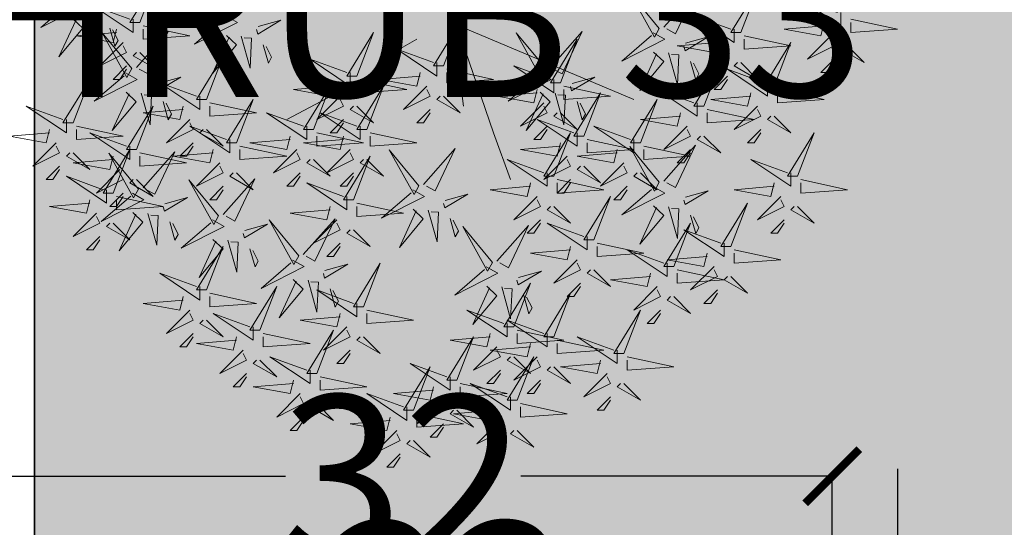
# Model space of a CAD drawing. Units: inches. Extents: x 1704 to 6393, y -157 to 1172.
# Tile 12 of 122: x 1898 to 1934, y 120 to 138. Entities that reach past the tile are written whole.
import ezdxf

# ---------------------------------------------------------------- set-up
doc = ezdxf.new("R2010")
doc.units = ezdxf.units.IN
doc.header["$MEASUREMENT"] = 0
for name, color, linetype, lineweight in [('A-ANNO-DIMS', 7, 'Continuous', 13), ('C-PROP', 7, 'Continuous', 35), ('L-shrub', 74, 'Continuous', 18)]:
    doc.layers.add(name, color=color, linetype=linetype, lineweight=lineweight)
doc.layers.add('L-PLNT-PATT', color=253, linetype='Continuous', lineweight=13, true_color=0x9abc8f)
doc.styles.get("Standard").update_dxf_attribs({"font": 'arial.ttf'})
doc.dimstyles.get("Standard").update_dxf_attribs({"dimtxt": 6, "dimasz": 2, "dimexe": 0.18, "dimexo": 0.0625, "dimgap": 0.09, "dimtad": 0, "dimtih": 1, "dimtoh": 1, "dimdec": 1, "dimzin": 0, "dimdsep": 46, "dimlunit": 3, "dimtxsty": 'Standard', "dimblk": 'ARCHTICK', "dimcen": 0.09, "dimadec": 0, "dimazin": 0, "dimtfac": 1, "dimtdec": 1, "dimtofl": 0, "dimtmove": 0, "dimatfit": 3, "dimfxl": 1, "dimtolj": 1, "dimtzin": 0, "dimarcsym": 0})

# ---------------------------------------------------------------- blocks, each defined once
blk = doc.blocks.new('autumn shrub')
at = {"layer": 'L-shrub'}
for p, q in [((11.54, 1.92), (51.94, 98)), ((71.18, 17.29), (98.12, 26.9)), ((9.62, -3.84), (71.18, 17.29)), ((11.54, -5.76), (55.79, 0)), ((17.31, -26.9), (25.01, -40.35)), ((46.17, -69.17), (63.49, -101.84))]:
    blk.add_line(p, q, dxfattribs=at)
for points in [[(5.77, 222.89), (11.54, 249.79), (13.47, 222.89), (7.7, 222.89)], [(21.16, 220.97), (30.78, 230.58), (23.09, 217.13), (21.16, 219.05)], [(1.92, 217.13), (9.62, 217.13), (-5.77, 194.07), (1.92, 215.21)], [(98.12, 194.07), (103.89, 220.97), (105.81, 194.07), (100.04, 194.07)], [(15.39, 211.36), (28.86, 197.91), (21.16, 213.28), (17.31, 211.36)], [(28.86, 213.28), (36.55, 205.6), (36.55, 209.44), (30.78, 213.28)], [(7.7, 207.52), (15.39, 205.6), (11.54, 184.46), (9.62, 207.52)], [(46.17, 180.62), (51.94, 207.52), (53.87, 180.62), (48.1, 180.62)], [(96.19, 192.15), (71.18, 201.75), (96.19, 186.38), (96.19, 192.15)], [(113.51, 192.15), (123.13, 201.75), (115.43, 188.3), (113.51, 190.23)], [(15.39, 161.4), (21.16, 188.3), (23.09, 161.4), (17.31, 161.4)], [(44.25, 178.7), (19.24, 188.3), (44.25, 172.93), (44.25, 178.7)], [(61.56, 178.7), (71.18, 188.3), (63.49, 174.85), (61.56, 176.78)], [(94.27, 188.3), (101.96, 188.3), (86.57, 165.25), (94.27, 186.38)], [(107.74, 182.54), (121.2, 169.09), (113.51, 184.46), (109.66, 182.54)], [(121.2, 184.46), (128.9, 176.78), (128.9, 180.62), (123.13, 184.46)], [(138.52, 155.64), (144.29, 182.54), (146.21, 155.64), (140.44, 155.64)], [(100.04, 178.7), (107.74, 176.78), (103.89, 155.64), (101.96, 178.7)], [(42.32, 174.85), (50.02, 174.85), (34.63, 151.8), (42.32, 172.93)], [(55.79, 169.09), (69.26, 155.64), (61.56, 171.01), (57.72, 169.09)], [(69.26, 171.01), (76.95, 163.33), (76.95, 167.17), (71.18, 171.01)], [(13.47, 159.48), (-11.54, 169.09), (13.47, 153.72), (13.47, 159.48)], [(30.78, 159.48), (40.4, 169.09), (32.71, 155.64), (30.78, 157.56)], [(48.1, 165.25), (55.79, 163.33), (51.94, 142.19), (50.02, 165.25)], [(57.72, 140.27), (63.49, 167.17), (65.41, 140.27), (59.64, 140.27)], [(136.59, 153.72), (111.58, 163.33), (136.59, 147.95), (136.59, 153.72)], [(153.91, 153.72), (163.53, 163.33), (155.83, 149.87), (153.91, 151.8)], [(11.54, 155.64), (19.24, 155.64), (3.85, 132.58), (11.54, 153.72)], [(25.01, 149.87), (38.48, 136.42), (30.78, 151.8), (26.93, 149.87)], [(55.79, 138.35), (30.78, 147.95), (55.79, 132.58), (55.79, 138.35)], [(38.48, 151.8), (46.17, 144.11), (46.17, 147.95), (40.4, 151.8)], [(73.11, 138.35), (82.73, 147.95), (75.03, 134.5), (73.11, 136.42)], [(134.67, 149.87), (142.36, 149.87), (126.97, 126.82), (134.67, 147.95)], [(150.06, 122.97), (155.83, 149.87), (157.76, 122.97), (151.98, 122.97)], [(17.31, 146.03), (25.01, 144.11), (21.16, 122.97), (19.24, 146.03)], [(148.14, 144.11), (161.6, 130.66), (153.91, 146.03), (150.06, 144.11)], [(161.6, 146.03), (169.3, 138.35), (169.3, 142.19), (163.53, 146.03)], [(19.67, 127.72), (16.03, 140.82), (23.96, 127.51), (21.35, 126.78)], [(108.17, 127.72), (104.53, 140.82), (112.46, 127.51), (109.84, 126.78)], [(140.44, 140.27), (148.14, 138.35), (144.29, 117.21), (142.36, 140.27)], [(10.44, 115.26), (-10.16, 133.5), (14.22, 121.96), (11.38, 116.94)], [(30.15, 130.65), (40.62, 133.58), (37.28, 135.46), (31.09, 132.32)], [(53.87, 134.5), (61.56, 134.5), (46.17, 111.45), (53.87, 132.58)], [(67.33, 128.74), (80.8, 115.29), (73.11, 130.66), (69.26, 128.74)], [(98.93, 115.26), (78.34, 133.5), (102.71, 121.96), (99.88, 116.94)], [(78.88, 103.76), (84.65, 130.66), (86.57, 103.76), (80.8, 103.76)], [(80.8, 130.66), (88.5, 122.97), (88.5, 126.82), (82.73, 130.66)], [(118.64, 130.65), (129.12, 133.58), (125.77, 135.46), (119.59, 132.32)], [(148.14, 121.05), (123.13, 130.66), (148.14, 115.29), (148.14, 121.05)], [(165.45, 121.05), (175.07, 130.66), (167.38, 117.21), (165.45, 119.13)], [(59.64, 124.9), (67.33, 122.97), (63.49, 101.84), (61.56, 124.9)], [(25.2, 117.98), (43.54, 123.1), (26.37, 123.95), (26.15, 119.65)], [(113.7, 117.98), (132.03, 123.1), (114.86, 123.95), (114.65, 119.65)], [(200.08, 94.15), (205.85, 121.05), (207.78, 94.15), (202, 94.15)], [(13.57, 109.08), (17.35, 115.78), (29.87, 91.05), (15.24, 108.13)], [(24.77, 109.38), (30.23, 115.14), (46.74, 101.41), (25.72, 111.06)], [(102.06, 109.08), (105.85, 115.78), (118.37, 91.05), (103.74, 108.13)], [(113.27, 109.38), (118.72, 115.14), (135.24, 101.41), (114.21, 111.06)], [(146.21, 117.21), (153.91, 117.21), (138.52, 94.15), (146.21, 115.29)], [(159.68, 111.45), (173.15, 98), (165.45, 113.37), (161.6, 111.45)], [(173.15, 113.37), (180.84, 105.68), (180.84, 109.52), (175.07, 113.37)], [(11.17, 112.64), (-9.49, 95.58), (16.19, 109.81), (11.17, 112.64)], [(76.95, 101.84), (51.94, 111.45), (76.95, 96.07), (76.95, 101.84)], [(99.66, 112.64), (79.01, 95.58), (104.68, 109.81), (99.66, 112.64)], [(94.27, 101.84), (103.89, 111.45), (96.19, 98), (94.27, 99.92)], [(134.67, 76.86), (140.44, 103.76), (142.36, 76.86), (136.59, 76.86)], [(151.98, 107.6), (159.68, 105.68), (155.83, 84.54), (153.91, 107.6)], [(75.03, 98), (82.73, 98), (67.33, 74.94), (75.03, 96.07)], [(75.03, 71.09), (80.8, 98), (82.73, 71.09), (76.95, 71.09)], [(198.16, 92.23), (173.15, 101.84), (198.16, 86.47), (198.16, 92.23)], [(215.47, 92.23), (225.09, 101.84), (217.4, 88.39), (215.47, 90.31)], [(88.5, 92.23), (101.96, 78.78), (94.27, 94.15), (90.42, 92.23)], [(101.96, 94.15), (109.66, 86.47), (109.66, 90.31), (103.89, 94.15)], [(80.8, 88.39), (88.5, 86.47), (84.65, 65.33), (82.73, 88.39)], [(196.23, 88.39), (203.93, 88.39), (188.54, 65.33), (196.23, 86.47)], [(44.25, 57.64), (50.02, 84.54), (51.94, 57.64), (46.17, 57.64)], [(98.12, 53.8), (103.89, 80.7), (105.81, 53.8), (100.04, 53.8)], [(132.75, 74.94), (107.74, 84.54), (132.75, 69.17), (132.75, 74.94)], [(150.06, 74.94), (159.68, 84.54), (151.98, 71.09), (150.06, 73.02)], [(190.46, 53.8), (196.23, 80.7), (198.16, 53.8), (192.39, 53.8)], [(209.7, 82.62), (223.17, 69.17), (215.47, 84.54), (211.62, 82.62)], [(223.17, 84.54), (230.86, 76.86), (230.86, 80.7), (225.09, 84.54)], [(42.76, 62.39), (39.12, 75.49), (47.05, 62.18), (44.43, 61.45)], [(73.11, 69.17), (48.1, 78.78), (73.11, 63.41), (73.11, 69.17)], [(90.42, 69.17), (100.04, 78.78), (92.34, 65.33), (90.42, 67.25)], [(202, 78.78), (209.7, 76.86), (205.85, 55.72), (203.93, 78.78)], [(33.52, 49.93), (12.93, 68.17), (37.3, 56.63), (34.47, 51.61)], [(53.23, 65.32), (63.71, 68.25), (60.36, 70.13), (54.18, 66.99)], [(130.82, 71.09), (138.52, 71.09), (123.13, 48.04), (130.82, 69.17)], [(42.32, 55.72), (17.31, 65.33), (42.32, 49.96), (42.32, 55.72)], [(59.64, 55.72), (69.26, 65.33), (61.56, 51.88), (59.64, 53.8)], [(71.18, 65.33), (78.88, 65.33), (63.49, 42.27), (71.18, 63.41)], [(144.29, 65.33), (157.76, 51.88), (150.06, 67.25), (146.21, 65.33)], [(157.76, 67.25), (165.45, 59.57), (165.45, 63.41), (159.68, 67.25)], [(48.29, 52.64), (66.62, 57.77), (49.45, 58.62), (49.24, 54.32)], [(96.19, 51.88), (71.18, 61.49), (96.19, 46.12), (96.19, 51.88)], [(84.65, 59.57), (98.12, 46.12), (90.42, 61.49), (86.57, 59.57)], [(98.12, 61.49), (105.81, 53.8), (105.81, 57.64), (100.04, 61.49)], [(113.51, 51.88), (123.13, 61.49), (115.43, 48.04), (113.51, 49.96)], [(136.59, 61.49), (144.29, 59.57), (140.44, 38.43), (138.52, 61.49)], [(188.54, 51.88), (163.53, 61.49), (188.54, 46.12), (188.54, 51.88)], [(184.69, 30.74), (190.46, 57.64), (192.39, 30.74), (186.61, 30.74)], [(205.85, 51.88), (215.47, 61.49), (207.78, 48.04), (205.85, 49.96)], [(227.01, 32.67), (232.79, 59.57), (234.71, 32.67), (228.94, 32.67)], [(40.4, 51.88), (48.1, 51.88), (32.71, 28.82), (40.4, 49.96)], [(76.95, 55.72), (84.65, 53.8), (80.8, 32.67), (78.88, 55.72)], [(34.25, 47.31), (13.6, 30.25), (39.27, 44.48), (34.25, 47.31)], [(36.65, 43.75), (40.43, 50.45), (52.96, 25.72), (38.33, 42.8)], [(47.86, 44.05), (53.31, 49.81), (69.83, 36.08), (48.8, 45.73)], [(53.87, 46.12), (67.33, 32.67), (59.64, 48.04), (55.79, 46.12)], [(67.33, 48.04), (75.03, 40.35), (75.03, 44.19), (69.26, 48.04)], [(94.27, 48.04), (101.96, 48.04), (86.57, 24.98), (94.27, 46.12)], [(186.61, 48.04), (194.31, 48.04), (178.92, 24.98), (186.61, 46.12)], [(46.17, 42.27), (53.87, 40.35), (50.02, 19.21), (48.1, 42.27)], [(107.74, 42.27), (121.2, 28.82), (113.51, 44.19), (109.66, 42.27)], [(121.2, 44.19), (128.9, 36.51), (128.9, 40.35), (123.13, 44.19)], [(154.34, 31.65), (150.7, 44.75), (158.63, 31.44), (156.02, 30.7)], [(200.08, 42.27), (213.55, 28.82), (205.85, 44.19), (202, 42.27)], [(225.09, 30.74), (200.08, 40.35), (225.09, 24.98), (225.09, 30.74)], [(213.55, 44.19), (221.24, 36.51), (221.24, 40.35), (215.47, 44.19)], [(242.41, 30.74), (252.02, 40.35), (244.33, 26.9), (242.41, 28.82)], [(100.04, 38.43), (107.74, 36.51), (103.89, 15.37), (101.96, 38.43)], [(145.11, 19.19), (124.51, 37.43), (148.89, 25.89), (146.05, 20.86)], [(182.77, 28.82), (157.76, 38.43), (182.77, 23.06), (182.77, 28.82)], [(164.82, 34.57), (175.29, 37.5), (171.94, 39.39), (165.76, 36.25)], [(192.39, 38.43), (200.08, 36.51), (196.23, 15.37), (194.31, 38.43)], [(200.08, 28.82), (209.7, 38.43), (202, 24.98), (200.08, 26.9)], [(159.87, 21.9), (178.21, 27.02), (161.04, 27.87), (160.82, 23.58)], [(180.84, 24.98), (188.54, 24.98), (173.15, 1.92), (180.84, 23.06)], [(223.17, 26.9), (230.86, 26.9), (215.47, 3.84), (223.17, 24.98)], [(215.47, -1.92), (221.24, 24.98), (223.17, -1.92), (217.4, -1.92)], [(236.63, 21.14), (250.1, 7.69), (242.41, 23.06), (238.56, 21.14)], [(250.1, 23.06), (257.8, 15.37), (257.8, 19.21), (252.02, 23.06)], [(34.63, -9.61), (40.4, 17.29), (42.32, -9.61), (36.55, -9.61)], [(148.24, 13), (152.02, 19.71), (164.54, -5.03), (149.91, 12.06)], [(159.44, 13.31), (164.89, 19.07), (181.41, 5.33), (160.39, 14.99)], [(194.31, 19.21), (207.78, 5.76), (200.08, 21.14), (196.23, 19.21)], [(207.78, 21.14), (215.47, 13.45), (215.47, 17.29), (209.7, 21.14)], [(228.94, 17.29), (236.63, 15.37), (232.79, -5.76), (230.86, 17.29)], [(145.83, 16.57), (125.18, -0.5), (150.86, 13.74), (145.83, 16.57)], [(186.61, 15.37), (194.31, 13.45), (190.46, -7.69), (188.54, 15.37)], [(213.55, -3.84), (188.54, 5.76), (213.55, -9.61), (213.55, -3.84)], [(230.86, -3.84), (240.48, 5.76), (232.79, -7.69), (230.86, -5.76)], [(110.09, -10.62), (106.45, 2.47), (114.39, -10.84), (111.77, -11.57)], [(232.79, -26.9), (238.56, 0), (240.48, -26.9), (234.71, -26.9)], [(32.71, -11.53), (7.7, -1.92), (32.71, -17.29), (32.71, -11.53)], [(50.02, -11.53), (59.64, -1.92), (51.94, -15.37), (50.02, -13.45)], [(100.86, -23.09), (80.26, -4.84), (104.64, -16.38), (101.8, -21.41)], [(120.57, -7.7), (131.04, -4.77), (127.7, -2.88), (121.51, -6.02)], [(211.62, -7.69), (219.32, -7.69), (203.93, -30.74), (211.62, -9.61)], [(30.78, -15.37), (38.48, -15.37), (23.09, -38.43), (30.78, -17.29)], [(115.63, -20.37), (133.96, -15.25), (116.79, -14.4), (116.57, -18.7)], [(225.09, -13.45), (238.56, -26.9), (230.86, -11.53), (227.01, -13.45)], [(238.56, -11.53), (246.25, -19.21), (246.25, -15.37), (240.48, -11.53)], [(44.25, -21.14), (57.72, -34.59), (50.02, -19.21), (46.17, -21.14)], [(57.72, -19.21), (65.41, -26.9), (65.41, -23.06), (59.64, -19.21)], [(103.99, -29.27), (107.77, -22.57), (120.29, -47.3), (105.66, -30.21)], [(230.86, -28.82), (205.85, -19.21), (230.86, -34.59), (230.86, -28.82)], [(217.4, -17.29), (225.09, -19.21), (221.24, -40.35), (219.32, -17.29)], [(248.18, -28.82), (257.8, -19.21), (250.1, -32.67), (248.18, -30.74)], [(36.55, -24.98), (44.25, -26.9), (40.4, -48.04), (38.48, -24.98)], [(71.18, -53.8), (76.95, -26.9), (78.88, -53.8), (73.11, -53.8)], [(101.59, -25.71), (80.93, -42.77), (106.61, -28.54), (101.59, -25.71)], [(115.19, -28.96), (120.65, -23.2), (137.17, -36.94), (116.14, -27.29)], [(40.4, -59.57), (46.17, -32.67), (48.1, -59.57), (42.32, -59.57)], [(173.15, -55.72), (178.92, -28.82), (180.84, -55.72), (175.07, -55.72)], [(228.94, -32.67), (236.63, -32.67), (221.24, -55.72), (228.94, -34.59)], [(111.58, -61.49), (117.35, -34.59), (119.28, -61.49), (113.51, -61.49)], [(242.41, -38.43), (255.87, -51.88), (248.18, -36.51), (244.33, -38.43)], [(255.87, -36.51), (263.57, -44.19), (263.57, -40.35), (257.8, -36.51)], [(234.71, -42.27), (242.41, -44.19), (238.56, -65.33), (236.63, -42.27)], [(69.26, -55.72), (44.25, -46.12), (69.26, -61.49), (69.26, -55.72)], [(86.57, -55.72), (96.19, -46.12), (88.5, -59.57), (86.57, -57.64)], [(171.22, -57.64), (146.21, -48.04), (171.22, -63.41), (171.22, -57.64)], [(188.54, -57.64), (198.16, -48.04), (190.46, -61.49), (188.54, -59.57)], [(38.48, -61.49), (13.47, -51.88), (38.48, -67.25), (38.48, -61.49)], [(55.79, -61.49), (65.41, -51.88), (57.72, -65.33), (55.79, -63.41)], [(109.66, -63.41), (84.65, -53.8), (109.66, -69.17), (109.66, -63.41)], [(126.97, -63.41), (136.59, -53.8), (128.9, -67.25), (126.97, -65.33)], [(211.62, -82.62), (217.4, -55.72), (219.32, -82.62), (213.55, -82.62)], [(67.33, -59.57), (75.03, -59.57), (59.64, -82.62), (67.33, -61.49)], [(71.18, -84.54), (76.95, -57.64), (78.88, -84.54), (73.11, -84.54)], [(169.3, -61.49), (176.99, -61.49), (161.6, -84.54), (169.3, -63.41)], [(36.55, -65.33), (44.25, -65.33), (28.86, -88.39), (36.55, -67.25)], [(80.8, -65.33), (94.27, -78.78), (86.57, -63.41), (82.73, -65.33)], [(94.27, -63.41), (101.96, -71.09), (101.96, -67.25), (96.19, -63.41)], [(107.74, -67.25), (115.43, -67.25), (100.04, -90.31), (107.74, -69.17)], [(150.49, -79.8), (146.85, -66.7), (154.79, -80.01), (152.17, -80.74)], [(182.77, -67.25), (196.23, -80.7), (188.54, -65.33), (184.69, -67.25)], [(196.23, -65.33), (203.93, -73.02), (203.93, -69.17), (198.16, -65.33)], [(50.02, -71.09), (63.49, -84.54), (55.79, -69.17), (51.94, -71.09)], [(63.49, -69.17), (71.18, -76.86), (71.18, -73.02), (65.41, -69.17)], [(73.11, -69.17), (80.8, -71.09), (76.95, -92.23), (75.03, -69.17)], [(121.2, -73.02), (134.67, -86.47), (126.97, -71.09), (123.13, -73.02)], [(134.67, -71.09), (142.36, -78.78), (142.36, -74.94), (136.59, -71.09)], [(160.97, -76.87), (171.44, -73.94), (168.1, -72.06), (161.91, -75.19)], [(175.07, -71.09), (182.77, -73.02), (178.92, -94.15), (176.99, -71.09)], [(42.32, -74.94), (50.02, -76.86), (46.17, -98), (44.25, -74.94)], [(69.26, -86.47), (44.25, -76.86), (69.26, -92.23), (69.26, -86.47)], [(86.57, -86.47), (96.19, -76.86), (88.5, -90.31), (86.57, -88.39)], [(113.51, -76.86), (121.2, -78.78), (117.35, -99.92), (115.43, -76.86)], [(141.26, -92.26), (120.66, -74.02), (145.04, -85.56), (142.2, -90.58)], [(209.7, -84.54), (184.69, -74.94), (209.7, -90.31), (209.7, -84.54)], [(227.01, -84.54), (236.63, -74.94), (228.94, -88.39), (227.01, -86.47)], [(156.03, -89.54), (174.36, -84.42), (157.19, -83.57), (156.97, -87.87)], [(67.33, -90.31), (75.03, -90.31), (59.64, -113.37), (67.33, -92.23)], [(186.61, -115.29), (192.39, -88.39), (194.31, -115.29), (188.54, -115.29)], [(207.78, -88.39), (215.47, -88.39), (200.08, -111.45), (207.78, -90.31)], [(80.8, -96.07), (94.27, -109.52), (86.57, -94.15), (82.73, -96.07)], [(94.27, -94.15), (101.96, -101.84), (101.96, -98), (96.19, -94.15)], [(141.99, -94.88), (121.33, -111.94), (147.01, -97.71), (141.99, -94.88)], [(144.39, -98.44), (148.17, -91.74), (160.69, -116.47), (146.06, -99.39)], [(155.59, -98.13), (161.05, -92.38), (177.57, -106.11), (156.54, -96.46)], [(221.24, -94.15), (234.71, -107.6), (227.01, -92.23), (223.17, -94.15)], [(234.71, -92.23), (242.41, -99.92), (242.41, -96.07), (236.63, -92.23)], [(73.11, -99.92), (80.8, -101.84), (76.95, -122.97), (75.03, -99.92)], [(78.88, -128.74), (84.65, -101.84), (86.57, -128.74), (80.8, -128.74)], [(213.55, -98), (221.24, -99.92), (217.4, -121.05), (215.47, -98)], [(10.05, -118.23), (6.41, -105.13), (14.35, -118.44), (11.73, -119.17)], [(184.69, -117.21), (159.68, -107.6), (184.69, -122.97), (184.69, -117.21)], [(202, -117.21), (211.62, -107.6), (203.93, -121.05), (202, -119.13)], [(20.53, -115.3), (31, -112.37), (27.66, -110.49), (21.47, -113.62)], [(127.41, -125.91), (123.77, -112.81), (131.7, -126.12), (129.08, -126.86)], [(137.88, -122.99), (148.36, -120.06), (145.01, -118.17), (138.83, -121.31)], [(15.59, -127.97), (33.92, -122.85), (16.75, -122), (16.53, -126.3)], [(76.95, -130.66), (51.94, -121.05), (76.95, -136.42), (76.95, -130.66)], [(53.87, -146.03), (59.64, -119.13), (61.56, -146.03), (55.79, -146.03)], [(94.27, -130.66), (103.89, -121.05), (96.19, -134.5), (94.27, -132.58)], [(118.17, -138.37), (97.58, -120.13), (121.95, -131.67), (119.12, -136.7)], [(163.53, -146.03), (169.3, -119.13), (171.22, -146.03), (165.45, -146.03)], [(182.77, -121.05), (190.46, -121.05), (175.07, -144.11), (182.77, -122.97)], [(3.95, -136.87), (7.73, -130.17), (20.25, -154.9), (5.62, -137.82)], [(132.94, -135.66), (151.27, -130.54), (134.1, -129.69), (133.89, -133.98)], [(196.23, -126.82), (209.7, -140.27), (202, -124.9), (198.16, -126.82)], [(209.7, -124.9), (217.4, -132.58), (217.4, -128.74), (211.62, -124.9)], [(1.55, -133.31), (-19.11, -150.37), (6.57, -136.14), (1.55, -133.31)], [(15.15, -136.56), (20.61, -130.81), (37.13, -144.54), (16.1, -134.89)], [(75.03, -134.5), (82.73, -134.5), (67.33, -157.56), (75.03, -136.42)], [(188.54, -130.66), (196.23, -132.58), (192.39, -153.72), (190.46, -130.66)], [(51.94, -147.95), (26.93, -138.35), (51.94, -153.72), (51.94, -147.95)], [(69.26, -147.95), (78.88, -138.35), (71.18, -151.8), (69.26, -149.87)], [(88.5, -140.27), (101.96, -153.72), (94.27, -138.35), (90.42, -140.27)], [(118.9, -140.99), (98.25, -158.06), (123.92, -143.83), (118.9, -140.99)], [(101.96, -138.35), (109.66, -146.03), (109.66, -142.19), (103.89, -138.35)], [(121.3, -144.56), (125.08, -137.85), (137.61, -162.59), (122.98, -145.5)], [(132.51, -144.25), (137.96, -138.49), (154.48, -152.23), (133.45, -142.57)], [(161.6, -147.95), (136.59, -138.35), (161.6, -153.72), (161.6, -147.95)], [(178.92, -147.95), (188.54, -138.35), (180.84, -151.8), (178.92, -149.87)], [(80.8, -144.11), (88.5, -146.03), (84.65, -167.17), (82.73, -144.11)], [(50.02, -151.8), (57.72, -151.8), (42.32, -174.85), (50.02, -153.72)], [(159.68, -151.8), (167.38, -151.8), (151.98, -174.85), (159.68, -153.72)], [(9.62, -184.46), (15.39, -157.56), (17.31, -184.46), (11.54, -184.46)], [(63.49, -157.56), (76.95, -171.01), (69.26, -155.64), (65.41, -157.56)], [(76.95, -155.64), (84.65, -163.33), (84.65, -159.48), (78.88, -155.64)], [(173.15, -157.56), (186.61, -171.01), (178.92, -155.64), (175.07, -157.56)], [(186.61, -155.64), (194.31, -163.33), (194.31, -159.48), (188.54, -155.64)], [(42.76, -175.87), (39.12, -162.77), (47.05, -176.08), (44.43, -176.81)], [(55.79, -161.4), (63.49, -163.33), (59.64, -184.46), (57.72, -161.4)], [(82.73, -186.38), (88.5, -159.48), (90.42, -186.38), (84.65, -186.38)], [(112.02, -172.03), (108.37, -158.93), (116.31, -172.24), (113.69, -172.97)], [(122.49, -169.1), (132.97, -166.17), (129.62, -164.29), (123.44, -167.43)], [(165.45, -161.4), (173.15, -163.33), (169.3, -184.46), (167.38, -161.4)], [(53.23, -172.94), (63.71, -170.02), (60.36, -168.13), (54.18, -171.27)], [(102.78, -184.49), (82.19, -166.25), (106.56, -177.79), (103.73, -182.81)], [(33.52, -188.33), (12.93, -170.09), (37.3, -181.63), (34.47, -186.66)], [(107.74, -199.83), (113.51, -172.93), (115.43, -199.83), (109.66, -199.83)], [(7.7, -186.38), (-17.31, -176.78), (7.7, -192.15), (7.7, -186.38)], [(25.01, -186.38), (34.63, -176.78), (26.93, -190.23), (25.01, -188.3)], [(48.29, -185.62), (66.62, -180.5), (49.45, -179.65), (49.24, -183.94)], [(80.8, -188.3), (55.79, -178.7), (80.8, -194.07), (80.8, -188.3)], [(98.12, -188.3), (107.74, -178.7), (100.04, -192.15), (98.12, -190.23)], [(117.55, -181.77), (135.88, -176.65), (118.71, -175.8), (118.49, -180.1)], [(105.91, -190.67), (109.69, -183.97), (122.21, -208.7), (107.59, -191.62)], [(117.12, -190.37), (122.57, -184.61), (139.09, -198.34), (118.06, -188.69)], [(5.77, -190.23), (13.47, -190.23), (-1.92, -213.28), (5.77, -192.15)], [(34.25, -190.95), (13.6, -208.02), (39.27, -193.78), (34.25, -190.95)], [(36.65, -194.52), (40.43, -187.81), (52.96, -212.55), (38.33, -195.46)], [(47.86, -194.21), (53.31, -188.45), (69.83, -202.19), (48.8, -192.53)], [(78.88, -192.15), (86.57, -192.15), (71.18, -215.21), (78.88, -194.07)], [(105.81, -201.75), (80.8, -192.15), (105.81, -207.52), (105.81, -201.75)], [(103.51, -187.11), (82.85, -204.17), (108.53, -189.94), (103.51, -187.11)], [(123.13, -201.75), (132.75, -192.15), (125.05, -205.6), (123.13, -203.68)], [(19.24, -195.99), (32.71, -209.44), (25.01, -194.07), (21.16, -195.99)], [(32.71, -194.07), (40.4, -201.75), (40.4, -197.91), (34.63, -194.07)], [(67.33, -222.89), (73.11, -195.99), (75.03, -222.89), (69.26, -222.89)], [(92.34, -197.91), (105.81, -211.36), (98.12, -195.99), (94.27, -197.91)], [(105.81, -195.99), (113.51, -203.68), (113.51, -199.83), (107.74, -195.99)], [(10.91, -203.69), (21.38, -200.76), (18.04, -198.87), (11.85, -202.01)], [(11.54, -199.83), (19.24, -201.75), (15.39, -222.89), (13.47, -199.83)], [(84.65, -201.75), (92.34, -203.68), (88.5, -224.81), (86.57, -201.75)], [(103.89, -205.6), (111.58, -205.6), (96.19, -228.66), (103.89, -207.52)], [(117.35, -211.36), (130.82, -224.81), (123.13, -209.44), (119.28, -211.36)], [(130.82, -209.44), (138.52, -217.13), (138.52, -213.28), (132.75, -209.44)], [(5.97, -216.36), (24.3, -211.24), (7.13, -210.39), (6.91, -214.69)], [(65.41, -224.81), (40.4, -215.21), (65.41, -230.58), (65.41, -224.81)], [(82.73, -224.81), (92.34, -215.21), (84.65, -228.66), (82.73, -226.73)], [(109.66, -215.21), (117.35, -217.13), (113.51, -238.26), (111.58, -215.21)], [(-5.67, -225.26), (-1.89, -218.56), (10.63, -243.29), (-4, -226.2)], [(5.53, -224.95), (10.99, -219.19), (27.51, -232.93), (6.48, -223.28)], [(63.49, -228.66), (71.18, -228.66), (55.79, -251.71), (63.49, -230.58)], [(76.95, -234.42), (90.42, -247.87), (82.73, -232.5), (78.88, -234.42)], [(90.42, -232.5), (98.12, -240.18), (98.12, -236.34), (92.34, -232.5)], [(69.26, -238.26), (76.95, -240.18), (73.11, -261.32), (71.18, -238.26)]]:
    blk.add_lwpolyline(points, dxfattribs=at)
blk = doc.blocks.new('_ArchTick')
at = {"color": 0, "linetype": 'ByBlock', "const_width": 0.15}
blk.add_lwpolyline([(-0.5, -0.5), (0.5, 0.5)], dxfattribs=at)
blk = doc.blocks.new('*D78')
at = {"layer": 'A-ANNO-DIMS', "color": 0, "lineweight": -2, "transparency": 16777216}
for p, q in [((1896.87, 155.246), (1891.743, 155.246)), ((1891.923, 155.246), (1891.923, 141.742)), ((1891.923, 121.849), (1891.923, 135.353)), ((1896.87, 121.849), (1891.743, 121.849))]:
    blk.add_line(p, q, dxfattribs=at)
at = {"layer": 'Defpoints', "color": 0, "lineweight": -3, "transparency": 16777216}
for p in [(1896.932, 155.246), (1891.923, 121.849), (1896.932, 121.849)]:
    blk.add_point(p, dxfattribs=at)
at = {"layer": 'A-ANNO-DIMS', "color": 0, "lineweight": -2, "transparency": 16777216, "xscale": 2, "yscale": 2, "zscale": 2}
for p, rotation in [((1891.923, 155.246), 90), ((1891.923, 121.849), 270)]:
    blk.add_blockref('_ArchTick', p, dxfattribs=dict(at, rotation=rotation))
at = {"layer": 'A-ANNO-DIMS', "color": 0, "transparency": 16777216, "insert": (1891.923, 138.547), "char_height": 6, "attachment_point": 5}
blk.add_mtext('\\A1;AUTUMN SHRUB 33', dxfattribs=at)
blk = doc.blocks.new('*D79')
at = {"layer": 'A-ANNO-DIMS', "color": 0, "lineweight": -2, "transparency": 16777216}
for p, q in [((1896.932, 121.786), (1896.932, 116.659)), ((1930.289, 121.786), (1930.289, 116.659)), ((1896.932, 116.839), (1909.225, 116.839)), ((1930.289, 116.839), (1917.996, 116.839))]:
    blk.add_line(p, q, dxfattribs=at)
at = {"layer": 'Defpoints', "color": 0, "lineweight": -3, "transparency": 16777216}
for p in [(1896.932, 121.849), (1930.289, 121.849), (1930.289, 116.839)]:
    blk.add_point(p, dxfattribs=at)
at = {"layer": 'A-ANNO-DIMS', "color": 0, "lineweight": -2, "transparency": 16777216, "xscale": 2, "yscale": 2, "zscale": 2, "rotation": 180}
blk.add_blockref('_ArchTick', (1896.932, 116.839), dxfattribs=at)
at = {"layer": 'A-ANNO-DIMS', "color": 0, "lineweight": -2, "transparency": 16777216, "xscale": 2, "yscale": 2, "zscale": 2}
blk.add_blockref('_ArchTick', (1930.289, 116.839), dxfattribs=at)
at = {"layer": 'A-ANNO-DIMS', "color": 0, "transparency": 16777216, "insert": (1913.611, 116.839), "char_height": 6, "attachment_point": 5}
blk.add_mtext('\\A1;33', dxfattribs=at)
blk = doc.blocks.new('*D83')
at = {"layer": 'A-ANNO-DIMS', "color": 0, "lineweight": -2, "transparency": 16777216}
for p, q in [((1896.102, 116.575), (1896.102, 121.691)), ((1896.102, 121.511), (1907.632, 121.511)), ((1927.871, 121.511), (1916.342, 121.511)), ((1927.871, 116.575), (1927.871, 121.691))]:
    blk.add_line(p, q, dxfattribs=at)
at = {"layer": 'Defpoints', "color": 0, "lineweight": -3, "transparency": 16777216}
for p in [(1927.871, 121.511), (1896.102, 116.512), (1927.871, 116.512)]:
    blk.add_point(p, dxfattribs=at)
at = {"layer": 'A-ANNO-DIMS', "color": 0, "lineweight": -2, "transparency": 16777216, "xscale": 2, "yscale": 2, "zscale": 2, "rotation": 180}
blk.add_blockref('_ArchTick', (1896.102, 121.511), dxfattribs=at)
at = {"layer": 'A-ANNO-DIMS', "color": 0, "lineweight": -2, "transparency": 16777216, "xscale": 2, "yscale": 2, "zscale": 2}
blk.add_blockref('_ArchTick', (1927.871, 121.511), dxfattribs=at)
at = {"layer": 'A-ANNO-DIMS', "color": 0, "transparency": 16777216, "insert": (1911.987, 121.511), "char_height": 6, "attachment_point": 5}
blk.add_mtext('\\A1;32', dxfattribs=at)
blk = doc.blocks.new('*D93')
at = {"layer": 'A-ANNO-DIMS', "color": 0, "lineweight": -2, "transparency": 16777216}
for p, q in [((2605.286, 895.213), (1829.698, 895.213)), ((1829.878, 895.213), (1829.878, 495.866)), ((1829.878, 90.213), (1829.878, 489.56)), ((2605.286, 90.213), (1829.698, 90.213))]:
    blk.add_line(p, q, dxfattribs=at)
at = {"layer": 'Defpoints', "color": 0, "lineweight": -3, "transparency": 16777216}
for p in [(2605.349, 895.213), (1829.878, 90.213), (2605.349, 90.213)]:
    blk.add_point(p, dxfattribs=at)
at = {"layer": 'A-ANNO-DIMS', "color": 0, "lineweight": -2, "transparency": 16777216, "xscale": 2, "yscale": 2, "zscale": 2}
for p, rotation in [((1829.878, 895.213), 90), ((1829.878, 90.213), 270)]:
    blk.add_blockref('_ArchTick', p, dxfattribs=dict(at, rotation=rotation))
at = {"layer": 'A-ANNO-DIMS', "color": 0, "transparency": 16777216, "insert": (1829.878, 492.713), "char_height": 6, "attachment_point": 5}
blk.add_mtext('\\A1;805', dxfattribs=at)

msp = doc.modelspace()

# ---------------------------------------------------------------- hatches: boundary and pattern name
at = {"layer": 'L-PLNT-PATT', "transparency": 33554643}
h = msp.add_hatch(color=256, dxfattribs=at)
h.dxf.hatch_style = 1
h.paths.add_polyline_path([(1975.349, 202.213), (1898.349, 202.213), (1898.349, -3.787), (1975.349, -3.787)])

# ---------------------------------------------------------------- linework, layer by layer
at = {"layer": 'C-PROP'}
msp.add_line((1898.349, -3.787), (1898.349, 1033.213), dxfattribs=at)

# ---------------------------------------------------------------- block references
at = {"layer": 'L-shrub', "xscale": 0.0642956299502212, "yscale": 0.0642956299502212, "zscale": 0.0642956299502212, "rotation": 270}
msp.add_blockref('autumn shrub', (1914.228, 138.795), dxfattribs=at)

# ---------------------------------------------------------------- dimensions: what is measured, and where the dimension line sits
at = {"layer": 'A-ANNO-DIMS'}
dim = msp.add_linear_dim(base=(1829.878, 90.213), p1=(2605.349, 895.213), p2=(2605.349, 90.213), angle=90, dimstyle='Standard', override={"dimdec": 0, "dimlfac": 1, "dimrnd": 0, "dimzin": 0, "dimdsep": 46, "dimlunit": 2}, dxfattribs=at)
dim.commit()
dim.dimension.update_dxf_attribs({"geometry": '*D93', "text_midpoint": (1829.878, 492.713)})
dim = msp.add_linear_dim(base=(1891.923, 121.849), p1=(1896.932, 155.246), p2=(1896.932, 121.849), angle=270, text='AUTUMN SHRUB <>', dimstyle='Standard', override={"dimdec": 0, "dimlfac": 1, "dimrnd": 0, "dimzin": 0, "dimdsep": 46, "dimlunit": 2}, dxfattribs=at)
dim.commit()
dim.dimension.update_dxf_attribs({"geometry": '*D78', "text_midpoint": (1891.923, 138.547)})
for base, p1, p2, picture, middle in [((1927.871, 121.511), (1896.102, 116.512), (1927.871, 116.512), '*D83', (1911.987, 121.511)), ((1930.289, 116.839), (1896.932, 121.849), (1930.289, 121.849), '*D79', (1913.611, 116.839))]:
    dim = msp.add_linear_dim(base=base, p1=p1, p2=p2, dimstyle='Standard', override={"dimdec": 0, "dimlfac": 1, "dimrnd": 0, "dimzin": 0, "dimdsep": 46, "dimlunit": 2}, dxfattribs=at)
    dim.commit()
    dim.dimension.update_dxf_attribs({"geometry": picture, "text_midpoint": middle})

doc.saveas('drawing.dxf')
